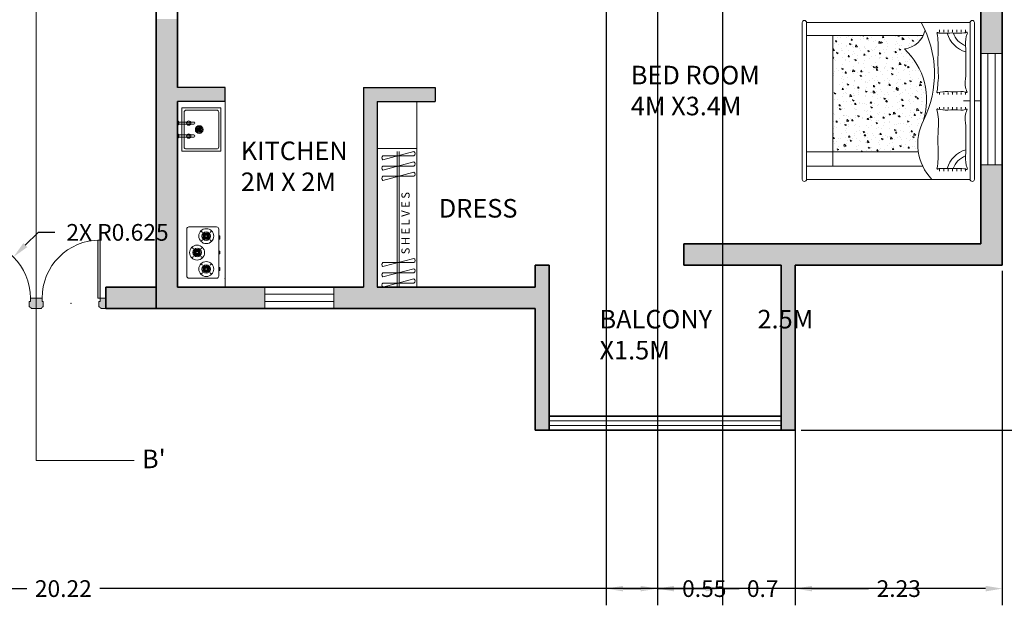
# Model space of a CAD drawing. Units: metres. Extents: x 2031 to 2061.8, y 1886.4 to 1909.8.
# Tile 7 of 10: x 2045.9 to 2056.5, y 1886.4 to 1892.7. Entities that reach past the tile are written whole.
import ezdxf

# ---------------------------------------------------------------- set-up
doc = ezdxf.new("R2010")
doc.units = ezdxf.units.M
for name, color, linetype, lineweight in [('A-ANNO-DIMS', 2, 'Continuous', 18), ('A-ANNO-SYMB', 7, 'Continuous', 18), ('A-AREA-IDEN', 7, 'Continuous', 18), ('A-EQPM', 8, 'Continuous', 18), ('A-FLOR-CASE', 8, 'Continuous', 18), ('A-FLOR-FIXT', 8, 'Continuous', 18), ('A-WALL-PATT', 252, 'Continuous', 13), ('doors & windows', 30, 'Continuous', 18), ('furniture', 24, 'Continuous', 13), ('grills', 5, 'Continuous', 13), ('inner walls', 4, 'Continuous', 25), ('windows', 30, 'Continuous', 18)]:
    doc.layers.add(name, color=color, linetype=linetype, lineweight=lineweight)
doc.layers.add('outer walls', color=1, linetype='Continuous', lineweight=35, plot=False)
doc.styles.get("Standard").update_dxf_attribs({"font": 'arial.ttf'})
doc.dimstyles.get("Standard").update_dxf_attribs({"dimtxt": 0.18, "dimasz": 0.18, "dimexe": 0.18, "dimexo": 0.0625, "dimgap": 0.09, "dimtad": 0, "dimtih": 1, "dimtoh": 1, "dimdec": 4, "dimzin": 0, "dimdsep": 46, "dimtxsty": 'Standard', "dimcen": 0.09, "dimadec": 0, "dimazin": 0, "dimtfac": 1, "dimtdec": 4, "dimtofl": 0, "dimtmove": 0, "dimatfit": 3, "dimfxl": 1, "dimtolj": 1, "dimtzin": 0, "dimarcsym": 0})

# ---------------------------------------------------------------- blocks, each defined once
blk = doc.blocks.new('sink')
for p, q in [((0, 0), (-22.00000000000001, 0)), ((0, 0), (0, 0)), ((-20.00000000000023, -2.999999999999995), (-2.000000000000178, -3)), ((-19.99999999999959, -22.99999999999988), (-20.00000000000023, -2.999999999999995)), ((-18.00000000000017, -3.999999999999996), (-4.000000000000113, -3.999999999999999)), ((-2.000000000000178, -3), (-1.999999999999543, -22.99999999999988)), ((-18.99999999999966, -20.99999999999994), (-19.00000000000017, -4.999999999999996)), ((-3.000000000000114, -5), (-2.999999999999607, -20.99999999999988)), ((-2.4e-15, -8.999999999999813), (-2.9e-15, -10.99999999999981)), ((-0.5000000000000026, -9.499999999999813), (-7.500000000000004, -9.499999999999812)), ((-0.5000000000000028, -10.49999999999981), (-7.500000000000004, -10.49999999999981)), ((-0.5000000000000026, -9.499999999999813), (-0.5000000000000028, -10.49999999999981)), ((-0.500000000000004, -15.49999999999981), (-7.500000000000005, -15.49999999999981)), ((-0.5000000000000044, -16.49999999999981), (-7.500000000000005, -16.49999999999981)), ((-0.500000000000004, -15.49999999999981), (-0.5000000000000044, -16.49999999999981)), ((-3.9e-15, -14.99999999999981), (-4.4e-15, -16.99999999999981)), ((-17.99999999999966, -21.99999999999988), (-3.999999999999607, -21.99999999999989)), ((-19.99999999999959, -22.99999999999988), (-1.999999999999543, -22.99999999999988))]:
    blk.add_line(p, q)
for centre, radius in [((-5.180961460384426, -9.999999999999812), 1), ((-10.00000000000014, -12.99999999999968), 1.794435724606955), ((-10.00000000000014, -12.99999999999968), 1.294435724606955), ((-10.66093109696162, -12.61841125325318), 0.25), ((-10.66093109696162, -13.38158874674618), 0.25), ((-10.00000000000014, -12.23682250650668), 0.25), ((-10.00000000000014, -12.99999999999968), 0.25), ((-10.00000000000014, -13.76317749349269), 0.25), ((-9.33906890303867, -12.61841125325318), 0.25), ((-9.33906890303867, -13.38158874674618), 0.25), ((-5.180961460384426, -9.999999999999812), 0.5), ((-5.180961460384427, -15.99999999999981), 1), ((-5.180961460384427, -15.99999999999981), 0.5)]:
    blk.add_circle(centre, radius)
for centre, radius, start, end in [((-18.00000000000017, -4.999999999999996), 1, 89.99999999999999, 180), ((-4.000000000000115, -5), 1, 0, 89.99999999999999), ((0.010449978117122, -9.510449978116938), 0.5105569333604445, 91.17280055555744, 178.8271994444424), ((-7.500000000000004, -9.999999999999812), 0.5, 89.99999999999999, 270), ((0.0104499781171218, -10.48955002188269), 0.5105569333604445, 181.1728005555574, 268.8271994444423), ((-7.500000000000005, -15.99999999999981), 0.5, 89.99999999999999, 270), ((0.0104499781171206, -15.51044997811693), 0.5105569333604445, 91.17280055555744, 178.8271994444424), ((0.0104499781171203, -16.48955002188269), 0.5105569333604445, 181.1728005555573, 268.8271994444423), ((-17.99999999999966, -20.99999999999988), 1, 180, 270), ((-3.999999999999607, -20.99999999999988), 1, 270, 0)]:
    blk.add_arc(centre, radius, start, end)
blk = doc.blocks.new('stove')
at = {"layer": 'furniture'}
h = blk.add_hatch(dxfattribs=at)
h.set_pattern_fill('HEX', color=256, angle=180, style=0)
h.set_pattern_definition([(360, (23.99999999999982, 24.99999999999816), (1e-16, 0.216506351), [0.125, -0.25]), (119.9999999999999, (23.99999999999982, 24.99999999999816), (-0.1875000000466704, -0.1082531754999999), [0.1249999999999998, -0.2499999999999996]), (59.99999999999994, (24.12499999999982, 24.99999999999816), (-0.1875000000466704, 0.1082531755000001), [0.125, -0.25])])
h.paths.add_polyline_path([(10.36428182591571, 19.71316705046143, 1), (7.364281825915714, 19.71316705046143, 1)])
h.paths.add_polyline_path([(9.364281825915715, 19.71316705046143, -1), (8.364281825915715, 19.71316705046143, -1)], flags=16)
h = blk.add_hatch(dxfattribs=at)
h.set_pattern_fill('HEX', color=256, angle=180, style=0)
h.set_pattern_definition([(180, (-2.000000000000001, 6.713167050462818), (-1e-16, -0.216506351), [0.125, -0.25]), (300, (-2.000000000000001, 6.713167050462818), (0.1875000000466704, 0.1082531754999999), [0.1249999999999999, -0.2499999999999998]), (239.9999999999999, (-2.125000000000001, 6.713167050462818), (0.1875000000466704, -0.1082531755000001), [0.125, -0.25])])
h.paths.add_polyline_path([(14.6357181740841, 11.99999999999954, 1), (11.6357181740841, 11.99999999999954, 1)])
h.paths.add_polyline_path([(12.6357181740841, 11.99999999999954, -1), (13.6357181740841, 11.99999999999954, -1)], flags=16)
h = blk.add_hatch(dxfattribs=at)
h.set_pattern_fill('HEX', color=256, angle=180, style=0)
h.set_pattern_definition([(360, (23.99999999999982, -0.9999999999999342), (-1e-16, -0.216506351), [0.125, -0.25]), (239.9999999999999, (23.99999999999982, -0.9999999999999342), (-0.1875000000466704, 0.1082531755), [0.1249999999999999, -0.2499999999999998]), (300, (24.12499999999982, -0.9999999999999342), (-0.1875000000466704, -0.1082531755), [0.125, -0.2499999999999999])])
h.paths.add_polyline_path([(10.36428182591571, 4.2868329495368, 1), (7.364281825915714, 4.2868329495368, 1)])
h.paths.add_polyline_path([(9.364281825915715, 4.2868329495368, -1), (8.364281825915715, 4.2868329495368, -1)], flags=16)
for p, q in [((4.000000000000007, 23.99999999999909), (17, 23.99999999999908)), ((3.000000000000007, 19.86017834974973), (2.500000000000003, 19.86017834974973)), ((2.500000000000003, 19.86017834974973), (2.500000000000003, 18.36017834974973)), ((3, 1.000000000000003), (3.000000000000007, 22.99999999999909)), ((6.389408091762671, 22.18804078461422), (7.09651487294905, 21.48093400342751)), ((10.6320487788818, 21.48093400342809), (11.33915556006851, 22.18804078461447)), ((18, 22.99999999999908), (18, 0.9999999999991327)), ((2.500000000000003, 18.36017834974973), (3.000000000000003, 18.36017834974973)), ((6.389408091762675, 17.23829331630864), (7.096514872949061, 17.94540009749535)), ((10.63204877888179, 17.94540009749477), (11.3391555600685, 17.23829331630838)), ((11.36795122111803, 13.7677669529662), (10.66084443993131, 14.47487373415259)), ((15.61059190823715, 14.47487373415233), (14.90348512705075, 13.76776695296562)), ((2.500000000000003, 12.64999999999954), (2.500000000000003, 11.34999999999955)), ((3.000000000000003, 12.64999999999954), (2.500000000000003, 12.64999999999954)), ((2.500000000000003, 11.34999999999955), (3.000000000000003, 11.34999999999955)), ((11.36795122111803, 10.23223304703288), (10.66084443993131, 9.525126265846504)), ((15.61059190823714, 9.525126265846753), (14.90348512705077, 10.23223304703346)), ((2.500000000000003, 4.936832949536799), (2.500000000000003, 3.636832949536802)), ((3.000000000000003, 4.936832949536799), (2.500000000000003, 4.936832949536799)), ((6.389408091762671, 6.761706683689592), (7.096514872949061, 6.054599902502877)), ((10.63204877888178, 6.05459990250346), (11.3391555600685, 6.761706683689842)), ((2.500000000000003, 3.636832949536802), (3.000000000000003, 3.636832949536802)), ((16.99999999999994, -8.669e-13), (3.999999999999946, 3.6e-15)), ((6.389408091762668, 1.811959215384014), (7.096514872949043, 2.519065996570723)), ((10.63204877888179, 2.519065996570138), (11.3391555600685, 1.81195921538376))]:
    blk.add_line(p, q, dxfattribs=at)
for centre, radius in [((8.864281825915715, 19.71316705046143), 3.499999999999999), ((8.864281825915715, 19.71316705046143), 1.999999999999999), ((8.864281825915715, 19.71316705046143), 1.5), ((8.864281825915715, 19.71316705046143), 0.5000000000000004), ((13.1357181740841, 11.99999999999954), 3.499999999999999), ((13.1357181740841, 11.99999999999954), 1.999999999999999), ((13.1357181740841, 11.99999999999954), 1.5), ((13.1357181740841, 11.99999999999954), 0.5000000000000004), ((8.864281825915715, 4.286832949536801), 3.499999999999999), ((8.864281825915715, 4.2868329495368), 1.999999999999999), ((8.864281825915715, 4.2868329495368), 1.5), ((8.864281825915715, 4.2868329495368), 0.5000000000000004)]:
    blk.add_circle(centre, radius, dxfattribs=at)
for centre, start, end in [((4.000000000000007, 22.99999999999909), 90, 180), ((17, 22.99999999999908), 0, 90), ((4, 1.000000000000003), 180, 269.9999999999968), ((17, 0.9999999999991331), 269.9999999999968, 0)]:
    blk.add_arc(centre, 1, start, end, dxfattribs=at)
at = {"layer": 'furniture', "ltscale": 9}
blk.add_point((0, 0), dxfattribs=at)
blk = doc.blocks.new('hangers')
at = {"layer": 'furniture'}
for p, q in [((1.8e-15, 16.5), (4.000000000000001, 1.5)), ((2.000000000000001, 16.5), (2.000000000000001, 1.5)), ((5.000000000000001, 16.5), (9.000000000000002, 1.5)), ((7.000000000000001, 16.5), (7.000000000000001, 1.5)), ((10, 16.5), (14, 1.5)), ((12, 16.5), (12, 1.5)), ((52, 16.5), (56, 1.5)), ((54, 16.5), (54, 1.5)), ((57, 16.5), (61, 1.5)), ((59, 16.5), (59, 1.5)), ((62, 16.5), (66, 1.5)), ((64, 16.5), (64, 1.5)), ((66, 9.5), (1.8e-15, 9.5)), ((1.8e-15, 8.5), (66, 8.5))]:
    blk.add_line(p, q, dxfattribs=at)
for centre, radius, start, end in [((1.000000000000001, 15.6218374153911), 1.33085293139661, 41.28839256573093, 138.711607434269), ((6.000000000000001, 15.6218374153911), 1.33085293139661, 41.28839256573093, 138.711607434269), ((11, 15.6218374153911), 1.33085293139661, 41.28839256573093, 138.711607434269), ((53, 15.6218374153911), 1.33085293139661, 41.28839256573107, 138.7116074342689), ((58, 15.6218374153911), 1.33085293139661, 41.28839256573107, 138.7116074342689), ((63, 15.6218374153911), 1.33085293139661, 41.28839256573107, 138.7116074342689), ((3.000000000000001, 1.915335972440686), 1.082822224561017, 202.5548696812492, 337.4451303187508), ((8.000000000000002, 1.915335972440686), 1.082822224561017, 202.5548696812492, 337.4451303187508), ((13, 1.915335972440686), 1.082822224561017, 202.5548696812492, 337.4451303187508), ((55, 1.915335972440686), 1.082822224561017, 202.5548696812491, 337.4451303187509), ((60, 1.915335972440686), 1.082822224561017, 202.5548696812491, 337.4451303187509), ((65, 1.915335972440686), 1.082822224561017, 202.5548696812491, 337.4451303187509)]:
    blk.add_arc(centre, radius, start, end, dxfattribs=at)
blk.add_point((0, 0), dxfattribs=at)
blk.add_text('S H E L V E S', height=4, dxfattribs=at).set_placement((15.9969173169515, 3.475366291579639))
blk = doc.blocks.new('bed')
at = {"layer": 'furniture'}
h = blk.add_hatch(dxfattribs=at)
h.set_pattern_fill('AR-CONC', color=256, angle=-90.00000000000003, style=0)
h.set_pattern_definition([(320, (0, 2.380000000001032), (-0.6275213498259539, -7.172601826007534), [0.75, -8.25]), (265, (0, 2.380000000001032), (7.521921337000119, 1.387513336129997), [0.6, -6.599999999999999]), (10.45139999999999, (-0.0522933999999964, 1.782283200001032), (6.894395420609534, -5.785093817140218), [0.6374019000000001, -7.011421119999999]), (316.1842, (2, 2.380000000001032), (-1.655190143290184, -10.67241048625644), [1.125, -12.375]), (6.635599999999979, (1.862066929999997, 1.490632550001038), (9.741178709004412, -9.346627055487035), [0.956102879999999, -10.51712999999998]), (261.1842, (2, 2.380000000001032), (9.741186009253243, -9.346619451336275), [0.8999999999999989, -9.899999999999984]), (291, (1.5, 1.380000000001032), (-4.02618890665339, -5.969070521184614), [0.75, -8.25]), (236, (1.5, 1.380000000001032), (7.251500450468529, -2.433153319215819), [0.6, -6.599999999999999]), (341.4514, (1.164483939999996, 0.8825776700010266), (3.22530496709952, -8.402226285814901), [0.6374019000000001, -7.011421119999999]), (307.4999999999999, (0, 2.380000000001032), (3.328938538313114, -0.121598553172908), [0, -6.519999999999999, 0, -6.7, 0, -6.625]), (277.5, (0, 2.380000000001032), (3.944117118823601, -2.630695374421487), [0, -3.819999999999999, 0, -6.37, 0, -2.524999999999999]), (237.5, (0, 4.610000000001036), (-0.2255487173438, -5.33822436172409), [0, -2.5, 0, -7.799999999999999, 0, -10.35]), (227.5, (0, 5.610000000001036), (1.001049823323174, -5.831861693423862), [0, -3.25, 0, -5.179999999999999, 0, -7.349999999999999])])
h.paths.add_polyline_path([(30.01221964123038, -67.99999999999999), (30.01221964123036, -26.4972098666525, 0.2630430180581192), (23.90476957024844, -35.1500155485824, 0.2934236934375176), (-9.177957282599145, -26.46678060096597, -0.1566832162072435), (-23.39221964123496, -28.71851562074189), (-23.39221964123494, -67.99999999999999)])
for p, q in [((0, -3), (0, 0)), ((36.01221964123033, -3), (-36.01221964123033, -3)), ((-36.01221964123033, -5.000000000000028), (-36.01221964123027, -80)), ((36.01221964123033, -5.000000000000042), (-36.01221964123033, -5.000000000000028)), ((-31.23716250644156, -7.067621994530554), (-32.23716250644157, -7.067621994530554)), ((-3.810600647213163, -7.067621994530554), (-2.810600647213163, -7.067621994530554)), ((0, -8.000000000000043), (0, -5.000000000000042)), ((3.894900133777696, -7.067621994530526), (2.894900133777696, -7.067621994530526)), ((31.62837541028949, -7.067621994530526), (32.62837541028949, -7.067621994530526)), ((36.01221964123039, -79.99999999999999), (36.01221964123033, -5.000000000000042)), ((-31.23716250644156, -9.067621994530555), (-32.23716250644157, -9.067621994530555)), ((-31.23716250644156, -11.06762199453055), (-32.23716250644157, -11.06762199453055)), ((-31.23716250644156, -13.06762199453055), (-32.23716250644157, -13.06762199453055)), ((-3.810600647213163, -9.067621994530555), (-2.810600647213163, -9.067621994530555)), ((-3.810600647213163, -11.06762199453055), (-2.810600647213163, -11.06762199453055)), ((-3.810600647213163, -13.06762199453055), (-2.810600647213163, -13.06762199453055)), ((3.894900133777696, -9.067621994530526), (2.894900133777696, -9.067621994530526)), ((3.894900133777696, -11.06762199453052), (2.894900133777696, -11.06762199453052)), ((3.894900133777696, -13.06762199453052), (2.894900133777696, -13.06762199453052)), ((31.62837541028949, -9.067621994530526), (32.62837541028949, -9.067621994530526)), ((31.62837541028949, -11.06762199453052), (32.62837541028949, -11.06762199453052)), ((31.62837541028949, -13.06762199453052), (32.62837541028949, -13.06762199453052)), ((-31.23716250644156, -15.06762199453055), (-32.23716250644157, -15.06762199453055)), ((-31.23716250644156, -17.06762199453055), (-32.23716250644157, -17.06762199453055)), ((-3.810600647213163, -15.06762199453055), (-2.810600647213163, -15.06762199453055)), ((-3.810600647213163, -17.06762199453055), (-2.810600647213163, -17.06762199453055)), ((3.894900133777696, -15.06762199453052), (2.894900133777696, -15.06762199453052)), ((3.894900133777696, -17.06762199453052), (2.894900133777696, -17.06762199453052)), ((31.62837541028949, -15.06762199453052), (32.62837541028949, -15.06762199453052)), ((31.62837541028949, -17.06762199453052), (32.62837541028949, -17.06762199453052)), ((-31.23716250644156, -19.06762199453055), (-32.23716250644157, -19.06762199453055)), ((-3.810600647213163, -19.06762199453055), (-2.810600647213163, -19.06762199453055)), ((3.894900133777696, -19.06762199453052), (2.894900133777696, -19.06762199453052)), ((31.62837541028949, -19.06762199453052), (32.62837541028949, -19.06762199453052)), ((-36.01221964123027, -80), (36.01221964123039, -79.99999999999997)), ((-36.01221964123027, -82), (36.01221964123039, -82))]:
    blk.add_line(p, q, dxfattribs=at)
at = {"layer": 'furniture', "ltscale": 5}
blk.add_line((-30.0122196412303, -26.65900214866815), (-30.01221964123028, -80), dxfattribs=at)
at = {"layer": 'furniture', "ltscale": 7}
blk.add_line((30.01221964123039, -79.99999999999999), (30.01221964123036, -26.4972098666525), dxfattribs=at)
at = {"layer": 'furniture', "ltscale": 0.3}
for p, q in [((-23.39221964123493, -80.00000000000003), (-23.39221964123496, -28.71851562074188)), ((-30.01221964123028, -67.99999999999999), (30.01221964123039, -67.99999999999999))]:
    blk.add_line(p, q, dxfattribs=at)
at = {"layer": 'furniture'}
for centre, radius, start, end in [((-35.95310404783035, -4.000000000000014), 1.001745802777857, 93.38313670775338, 266.6168632922466), ((35.95310404783047, -4.000000000000014), 1.001745802777857, 273.3831367077534, 86.61686329224663), ((-31.09685452420217, -6.56812628935117), 0.3815901177143176, 35.89755946985184, 208.6271807330242), ((-44.4434251214767, -13.85312857714783), 14.82374463825802, 27.16285943351717, 28.62718073212637), ((-46.75951437957865, -9.65138206848897), 15.71579241958107, 357.4803608088326, 9.395608387614068), ((-34.45294545533051, -3.506108501804959), 9.853247350176973, 289.8695209624031, 338.9842964810487), ((-34.45294545533051, -3.506108501804959), 12.47479548168961, 286.0319050224358, 344.1205283884622), ((-26.34909713879518, 6.677823774407073), 13.75788850886336, 251.1782289026713, 273.3982224065857), ((-18.01528168092849, -163.5963416214672), 156.7209082093599, 87.00321809951629, 92.74968346925495), ((-8.031939823939297, 2.030581047412752), 9.294330538692307, 258.8960367609226, 294.7184225587751), ((0.254091396095987, -8.800915214962217), 4.494229367051207, 159.014640107615, 186.2730421081171), ((-4.029449448298862, -6.668977911985379), 0.2818061021667602, 335.7259061638442, 114.3030308467571), ((3.223958981487498, -9.94006998173215), 7.675076275868892, 155.7259061638442, 159.0146401085631), ((4.113748934860268, -6.668977911985379), 0.2818061021635516, 65.69696915417202, 204.2740938370052), ((-3.139659494904833, -9.940069981732137), 7.675076275868892, 20.98535989143595, 24.27409383615427), ((-0.1697919095242355, -8.800915214962217), 4.494229367051207, 353.7269578918828, 20.98535989238499), ((8.116239310533615, 2.030581047735168), 9.294330539002221, 245.2815774418415, 281.1039632384965), ((18.09958116748922, -163.5963416214399), 156.7209082093326, 87.2503165307418, 92.99678190048373), ((34.53724494190226, -3.506108501789682), 12.47479548168961, 195.8794716115377, 253.9680949775642), ((34.53724494190226, -3.506108501789682), 9.853247350176973, 201.0157035189505, 250.1304790375968), ((26.43339662535652, 6.677823774423444), 13.75788850886336, 266.6017775934111, 288.8217710973251), ((31.18115401076358, -6.568126289351184), 0.3815901177179044, 331.3728192669758, 144.1024405301472), ((46.84381386614001, -9.651382068520647), 15.71579241958353, 170.6043916115409, 182.5196391911672), ((44.52772460803806, -13.85312857714784), 14.82374463825802, 151.3728192678729, 152.8371405664821), ((-28.61556435462791, 31.03444768063454), 42.31456350822244, 266.4835611990511, 266.6487421238194), ((54.88285648445511, -13.16191061182081), 85.98801403775587, 178.1208768196816, 183.3613129440673), ((-32.81622258778788, -12.43616332427339), 28.77528664700029, 354.3784002715227, 6.27304210895588), ((32.90052207435963, -12.43616332427341), 28.77528664700055, 173.7269578910441, 185.6215997284773), ((-54.79855699787332, -13.1619106118885), 85.98801403775471, 356.6386870559327, 1.87912318031836), ((28.69986384117891, 31.03444768073385), 42.31456350831875, 273.3512578762066, 273.5164388009489), ((12.27920019974715, -16.10835590841725), 16.48064095036883, 177.0317121189266, 192.8677860199701), ((-12.19490071317551, -16.10835590841725), 16.48064095036894, 347.1322139800299, 2.968287881073314), ((-19.78970084288576, -5.469494448941333), 23.52647715105876, 226.4060518471351, 297.4441169484015), ((-31.05019458355673, -19.91479358257859), 0.2912925215689113, 147.6219291273817, 311.93432899363), ((-33.19532486499685, -18.55460390606353), 2.248727139855352, 327.6219291288709, 339.224552802207), ((-34.12771521855714, -18.41167218428833), 3.177308659740759, 342.7808628527732, 3.755021134780372), ((-24.39731400277299, -58.0065508966982), 38.42172354635978, 93.51643880178425, 99.67664784205135), ((-24.51665474671893, -56.06449133928439), 36.47600066328987, 86.48356119821578, 93.51643880178425), ((-18.48842024981553, 70.49496359167773), 90.23180174042126, 267.5920770069633, 273.6328801943956), ((-10.30534078399284, -44.95285539311296), 25.51674577343078, 75.95197577712642, 95.54518109318596), ((12.50744191168894, -69.71437404891591), 48.3828132966499, 60.93454900685955, 116.3226601669859), ((-3.947726608991956, -19.99033763805275), 0.2654728058058112, 231.9004795059564, 52.89022406852256), ((4.032026095563765, -19.99033763805275), 0.2654728058058112, 127.1097759314774, 308.0995204940429), ((7.570216687580227, -34.67789736270967), 14.86666553287629, 87.39755039330738, 103.1191401867811), ((11.43897390287765, -34.80624327566366), 15.31635237680183, 84.69404282866213, 102.035481886755), ((18.57271973638731, 70.4949635916777), 90.23180174042125, 266.3671198056044, 272.4079229930367), ((24.6009542333012, -56.0644913392844), 36.47600066328987, 86.48356119821578, 93.51643880178425), ((24.48161348934542, -58.00655089669821), 38.42172354635978, 80.32335215794863, 86.48356119821578), ((31.13449407013883, -19.91479358255678), 0.2912925215689113, 228.06567100637, 32.37807087261824), ((34.21201470513921, -18.41167218428845), 3.177308659740705, 176.2449788652196, 197.2191371472267), ((33.27962435157895, -18.55460390604825), 2.248727139855352, 200.775447197793, 212.378070871129), ((0.602167516954296, -56.56840710701565), 31.65057281321388, 42.58740832788977, 108.5033645785765), ((34.6132349005153, -36.22659364526982), 10.76244628919441, 101.1719081394, 174.2590453022261), ((-35.95310404783035, -81), 1.001745802777857, 93.38313670775338, 266.6168632922466), ((35.95310404783044, -81), 1.001745802777857, 273.3831367077534, 86.61686329224663)]:
    blk.add_arc(centre, radius, start, end, dxfattribs=at)
blk = doc.blocks.new('D2')
at = {"layer": 'doors & windows'}
h = blk.add_hatch(dxfattribs=at)
h.set_pattern_fill('DOTS', color=256, scale=2, angle=180, style=0)
h.set_pattern_definition([(180, (0, -3.999999999998181), (-0.0625, -0.125), [0, -0.125])])
h.paths.add_polyline_path([(2.5, 1.819e-12), (3.5, 1.819e-12), (3.500000000001818, 24.97999199359535, 0.0100030022021123), (2.500000000001818, 25.00000000000182)])
h = blk.add_hatch(dxfattribs=at)
h.set_pattern_fill('DOTS', color=256, scale=2, angle=180, style=0)
h.set_pattern_definition([(180, (0, 0), (-0.0625, -0.125), [0, -0.125])])
edge = h.paths.add_edge_path()
edge.add_line((27.50000000000182, 1.819e-12), (27.50000000000182, -1.499999999998181))
edge.add_line((27.50000000000182, -1.499999999998181), (27.00000000000157, -1.499999999998181))
edge.add_line((27.00000000000157, -1.499999999998181), (27.00000000000039, -3.749999999998181))
edge.add_line((27.00000000000039, -3.749999999998181), (27.25, -3.749999999998181))
edge.add_arc((27.75893604593965, -3.741063954058532), 0.5090144907305875, 181.0059124648427, 268.9940875351573)
edge.add_line((27.75, -4.249999999998181), (27.75, -4.499999999998181))
edge.add_line((27.75, -4.499999999998181), (30.00000000000182, -4.499999999998181))
edge.add_line((30.00000000000182, -4.499999999998181), (30.00000000000182, 0))
edge.add_line((30.00000000000182, 0), (27.50000000000182, 1.819e-12))
edge = h.paths.add_edge_path()
edge.add_line((2.5, -1.499999999998181), (2.5, 1.819e-12))
edge.add_line((2.5, 1.819e-12), (1.819e-12, 0))
edge.add_line((1.819e-12, 0), (0, -4.499999999998181))
edge.add_line((0, -4.499999999998181), (2.250000000001548, -4.499999999998181))
edge.add_line((2.250000000001548, -4.499999999998181), (2.250000000001548, -4.249999999998181))
edge.add_arc((2.2410639540619, -3.741063954058532), 0.5090144907305875, 271.0059124648427, 358.9940875351573)
edge.add_line((2.750000000001548, -3.749999999998181), (3, -3.749999999998181))
edge.add_line((3, -3.749999999998181), (3, -1.499999999998181))
edge.add_line((3, -1.499999999998181), (2.5, -1.499999999998181))
for p, q in [((1.819e-12, 0), (0, -4.499999999998181)), ((30.00000000000182, 0), (30.00000000000182, -4.499999999998181))]:
    blk.add_line(p, q)
blk.add_lwpolyline([(3.5, 1.819e-12), (3.500000000001818, 25.00000000000182), (2.500000000001818, 25.00000000000182), (2.5, 1.819e-12)], close=True, dxfattribs=at)
for points in [[(3, -3.749999999998181), (3, -1.499999999998181), (2.5, -1.499999999998181), (2.5, 1.819e-12), (1.819e-12, 0)], [(27.00000000000039, -3.749999999998181), (27.00000000000182, -1.499999999998181), (27.50000000000182, -1.499999999998181), (27.50000000000182, 1.819e-12), (30, 0)], [(0, -4.499999999998181), (2.250000000001548, -4.499999999998181)], [(30, -4.499999999998181), (27.75, -4.499999999998181)]]:
    blk.add_lwpolyline(points, dxfattribs=at)
for points in [[(2.250000000001548, -4.499999999998181), (2.250000000001548, -4.249999999998181, 0.4039662087126686), (2.750000000001548, -3.749999999998181), (3.000000000001548, -3.749999999998181)], [(27.75, -4.499999999998181), (27.75, -4.249999999998181, -0.4039662087126686), (27.25, -3.749999999998181), (27, -3.749999999998181)]]:
    blk.add_lwpolyline(points, format="xyb", dxfattribs=at)
at = {"layer": 'doors & windows', "ltscale": 6}
blk.add_arc((2.5, 1.819e-12), 25, 0, 90, dxfattribs=at)
at = {"layer": 'doors & windows'}
blk.add_point((15, -2.24999999999909), dxfattribs=at)
blk = doc.blocks.new('WIN-1200')
for p, q in [((0.2299999999995634, 1.200000000000045), (-4.547e-13, 1.199999999999818)), ((0.0750000000007276, -2.274e-13), (0.0749999999995907, 1.200000000000045)), ((0.1550000000006548, -2.274e-13), (0.154999999999518, 1.200000000000045)), ((0.2300000000007003, 0), (6.821e-13, -2.274e-13))]:
    blk.add_line(p, q)
blk = doc.blocks.new('BALCONY-GUARD-2500')
for p, q in [((4.547e-13, 0.0500000000010914), (2.5, 0.0500000000006367)), ((4.547e-13, 6.821e-13), (2.5, 4.547e-13))]:
    blk.add_line(p, q)
blk = doc.blocks.new('*D44')
at = {"layer": 'A-ANNO-DIMS', "color": 0, "lineweight": -2, "transparency": 16777216}
for p, q in [((2036.232783, 1900.719895), (2036.232783, 1886.390195)), ((2056.453886, 1889.9931), (2056.453886, 1886.390195)), ((2036.412783, 1886.570195), (2045.94901662824, 1886.570195)), ((2056.273886, 1886.570195), (2046.73765237176, 1886.570195))]:
    blk.add_line(p, q, dxfattribs=at)
at = {"layer": 'A-ANNO-DIMS', "color": 0, "transparency": 16777216}
for points in [[(2036.412783, 1886.600195), (2036.412783, 1886.540195), (2036.232783, 1886.570195)], [(2056.273886, 1886.600195), (2056.273886, 1886.540195), (2056.453886, 1886.570195)]]:
    blk.add_solid(points, dxfattribs=at)
at = {"layer": 'Defpoints', "color": 0, "transparency": 16777216}
for p in [(2036.232783, 1900.782395), (2056.453886, 1890.0556), (2056.453886, 1886.570195)]:
    blk.add_point(p, dxfattribs=at)
at = {"layer": 'A-ANNO-DIMS', "color": 0, "transparency": 16777216, "insert": (2046.3433345, 1886.570195), "char_height": 0.18, "attachment_point": 5}
blk.add_mtext('\\A1;20.22', dxfattribs=at)
blk = doc.blocks.new('*D45')
at = {"layer": 'A-ANNO-DIMS', "color": 0, "lineweight": -2, "transparency": 16777216}
for p, q in [((2047.556386000001, 1907.081203000001), (2061.614374000002, 1907.081203000001)), ((2061.434374000002, 1906.901203000001), (2061.434374000002, 1897.862029637791)), ((2061.434374000002, 1888.459050000001), (2061.434374000002, 1897.498223362211)), ((2054.286386000001, 1888.279050000001), (2061.614374000002, 1888.279050000001))]:
    blk.add_line(p, q, dxfattribs=at)
at = {"layer": 'A-ANNO-DIMS', "color": 0, "transparency": 16777216}
for points in [[(2061.404374000002, 1906.901203000001), (2061.464374000002, 1906.901203000001), (2061.434374000002, 1907.081203000001)], [(2061.404374000002, 1888.459050000001), (2061.464374000002, 1888.459050000001), (2061.434374000002, 1888.279050000001)]]:
    blk.add_solid(points, dxfattribs=at)
at = {"layer": 'Defpoints', "color": 0, "transparency": 16777216}
for p in [(2047.493886000001, 1907.081203000001), (2061.434374000002, 1907.081203000001), (2054.223886000001, 1888.279050000001)]:
    blk.add_point(p, dxfattribs=at)
at = {"layer": 'A-ANNO-DIMS', "color": 0, "transparency": 16777216, "insert": (2061.434374000002, 1897.6801265), "char_height": 0.18, "attachment_point": 5}
blk.add_mtext('\\A1;18.802', dxfattribs=at)
blk = doc.blocks.new('*D56')
at = {"layer": 'A-ANNO-DIMS', "color": 0, "lineweight": -2, "transparency": 16777216}
for p, q in [((2054.223886, 1889.9931), (2054.223886, 1886.390195)), ((2056.453886, 1889.9931), (2056.453886, 1886.390195)), ((2054.403886, 1886.570195), (2055.013572221009, 1886.570195)), ((2056.273886, 1886.570195), (2055.664199778991, 1886.570195))]:
    blk.add_line(p, q, dxfattribs=at)
at = {"layer": 'A-ANNO-DIMS', "color": 0, "transparency": 16777216}
for points in [[(2054.403886, 1886.600195), (2054.403886, 1886.540195), (2054.223886, 1886.570195)], [(2056.273886, 1886.600195), (2056.273886, 1886.540195), (2056.453886, 1886.570195)]]:
    blk.add_solid(points, dxfattribs=at)
at = {"layer": 'Defpoints', "color": 0, "transparency": 16777216}
for p in [(2054.223886, 1890.0556), (2056.453886, 1890.0556), (2056.453886, 1886.570195)]:
    blk.add_point(p, dxfattribs=at)
at = {"layer": 'A-ANNO-DIMS', "color": 0, "transparency": 16777216, "insert": (2055.338886, 1886.570195), "char_height": 0.18, "attachment_point": 5}
blk.add_mtext('\\A1;2.23', dxfattribs=at)
blk = doc.blocks.new('*D62')
at = {"layer": 'A-ANNO-DIMS', "color": 0, "lineweight": -2, "transparency": 16777216}
for p, q in [((2052.190038, 1893.772326), (2052.190038, 1886.390195)), ((2052.740231, 1893.6231), (2052.740231, 1886.390195)), ((2052.370038, 1886.570195), (2052.560231000001, 1886.570195)), ((2052.740231, 1886.570195), (2052.920231, 1886.570195))]:
    blk.add_line(p, q, dxfattribs=at)
at = {"layer": 'A-ANNO-DIMS', "color": 0, "transparency": 16777216}
for points in [[(2052.370038, 1886.600195), (2052.370038, 1886.540195), (2052.190038, 1886.570195)], [(2052.560231000001, 1886.600195), (2052.560231000001, 1886.540195), (2052.740231, 1886.570195)]]:
    blk.add_solid(points, dxfattribs=at)
at = {"layer": 'Defpoints', "color": 0, "transparency": 16777216}
for p in [(2052.190038, 1893.834826), (2052.740231, 1893.6856), (2052.740231, 1886.570195)]:
    blk.add_point(p, dxfattribs=at)
at = {"layer": 'A-ANNO-DIMS', "color": 0, "transparency": 16777216, "insert": (2053.244685297408, 1886.570195), "char_height": 0.18, "attachment_point": 5}
blk.add_mtext('\\A1;0.55', dxfattribs=at)
blk = doc.blocks.new('*D63')
at = {"layer": 'A-ANNO-DIMS', "color": 0, "lineweight": -2, "transparency": 16777216}
for p, q in [((2052.740231, 1893.6231), (2052.740231, 1886.390195)), ((2053.440231, 1893.623873), (2053.440231, 1886.390195)), ((2052.920231, 1886.570195), (2053.260231, 1886.570195)), ((2053.440231, 1886.570195), (2053.620231, 1886.570195))]:
    blk.add_line(p, q, dxfattribs=at)
at = {"layer": 'A-ANNO-DIMS', "color": 0, "transparency": 16777216}
for points in [[(2052.920231, 1886.600195), (2052.920231, 1886.540195), (2052.740231, 1886.570195)], [(2053.260231, 1886.600195), (2053.260231, 1886.540195), (2053.440231, 1886.570195)]]:
    blk.add_solid(points, dxfattribs=at)
at = {"layer": 'Defpoints', "color": 0, "transparency": 16777216}
for p in [(2052.740231, 1893.6856), (2053.440231, 1893.686373), (2053.440231, 1886.570195)]:
    blk.add_point(p, dxfattribs=at)
at = {"layer": 'A-ANNO-DIMS', "color": 0, "transparency": 16777216, "insert": (2053.874085024557, 1886.570195), "char_height": 0.18, "attachment_point": 5}
blk.add_mtext('\\A1;0.7', dxfattribs=at)
blk = doc.blocks.new('*D65')
at = {"layer": 'A-ANNO-DIMS', "color": 0, "lineweight": -2, "transparency": 16777216}
for p, q in [((2046.070887774461, 1890.408268174999), (2045.933100891741, 1890.270283483999)), ((2046.250887774462, 1890.408268174999), (2046.070887774461, 1890.408268174999)), ((2045.364289, 1889.610655), (2045.364289000001, 1889.790655)), ((2045.274289, 1889.700655), (2045.454289, 1889.700655))]:
    blk.add_line(p, q, dxfattribs=at)
at = {"layer": 'A-ANNO-DIMS', "color": 0, "transparency": 16777216}
blk.add_solid([(2045.911872477741, 1890.291481465956), (2045.954329305741, 1890.249085502042), (2045.805913, 1890.142913)], dxfattribs=at)
at = {"layer": 'Defpoints', "color": 0, "transparency": 16777216}
for p in [(2045.805913, 1890.142913), (2045.364289, 1889.700655)]:
    blk.add_point(p, dxfattribs=at)
at = {"layer": 'A-ANNO-DIMS', "color": 0, "transparency": 16777216, "insert": (2046.926317515253, 1890.408268174999), "char_height": 0.18, "attachment_point": 5}
blk.add_mtext('\\A1;2X R0.625', dxfattribs=at)

msp = doc.modelspace()

# ---------------------------------------------------------------- hatches: boundary and pattern name
at = {"layer": 'A-WALL-PATT'}
h = msp.add_hatch(color=256, dxfattribs=at)
h.dxf.hatch_style = 1
h.paths.add_polyline_path([(2051.57388605158, 1890.055599700484), (2051.42388605158, 1890.055599700485), (2051.42388605158, 1889.818154600064), (2049.72388605158, 1889.818154600064), (2049.72388605158, 1891.818397054436), (2050.347309493104, 1891.818397054436), (2050.347309493104, 1891.968397054436), (2049.573886051581, 1891.968397054436), (2049.573886051581, 1889.818154600064), (2049.254524170275, 1889.818154600064), (2049.254524170275, 1889.588154600064), (2051.42388605158, 1889.588154600064), (2051.42388605158, 1888.279049770338), (2051.57388605158, 1888.279049770338)])
h.paths.add_polyline_path([(2048.511176543873, 1889.818154600065), (2047.57388605158, 1889.818154600065), (2047.573886051581, 1891.818397054435), (2048.085735884881, 1891.818397054435), (2048.085735884881, 1891.968397054435), (2047.573886051581, 1891.968397054435), (2047.57388605158, 1892.707982727461), (2047.343886051579, 1892.707982727461), (2047.343886051578, 1889.588154600065), (2048.511176543873, 1889.588154600065)])
h.paths.add_polyline_path([(2047.57388605158, 1895.334826264002), (2047.57388605158, 1895.571212564149), (2047.34388605158, 1895.571212564149), (2047.343886051579, 1893.707982727461), (2047.57388605158, 1893.707982727461)])
h = msp.add_hatch(color=256, dxfattribs=at)
h.dxf.hatch_style = 1
h.paths.add_polyline_path([(2056.45388605158, 1891.13542096002), (2056.223886051581, 1891.13542096002), (2056.223886051581, 1890.285599700484), (2053.026296602634, 1890.285599700484), (2053.026296602634, 1890.055599700484), (2054.07388605158, 1890.055599700484), (2054.07388605158, 1888.279049770337), (2054.22388605158, 1888.279049770337), (2054.22388605158, 1890.055599700484), (2056.45388605158, 1890.055599700484)])
h.paths.add_polyline_path([(2056.45388605158, 1893.915599700484), (2054.920037956281, 1893.915599700483), (2054.920037956281, 1893.685599700484), (2056.223886051581, 1893.685599700484), (2056.223886051581, 1892.33542096002), (2056.45388605158, 1892.33542096002)])
h = msp.add_hatch(color=256, dxfattribs=at)
h.dxf.hatch_style = 1
h.paths.add_polyline_path([(2047.343886051578, 1889.818154600065), (2046.801788731911, 1889.818154600065), (2046.801788731911, 1889.588154600065), (2047.343886051578, 1889.588154600065)])

# ---------------------------------------------------------------- linework, layer by layer
at = {"layer": 'A-ANNO-SYMB'}
for q in [(2046.051788731911, 1908.279650182242), (2046.051788731911, 1887.95119549084), (2047.107009925013, 1887.95119549084)]:
    msp.add_line((2046.051788731911, 1887.95119549084), q, dxfattribs=at)
at = {"layer": 'A-FLOR-CASE', "ltscale": 0.3}
for p, q in [((2048.085735884882, 1889.818154600065), (2048.085735884881, 1891.818397054435)), ((2050.149066122807, 1889.818154600066), (2050.149066122807, 1891.818397054436))]:
    msp.add_line(p, q, dxfattribs=at)
at = {"layer": 'A-FLOR-CASE'}
msp.add_line((2050.149066122807, 1891.311337225385), (2049.72388605158, 1891.311337225385), dxfattribs=at)
at = {"layer": 'inner walls'}
for p, q in [((2048.085735884881, 1891.968397054435), (2047.57388605158, 1891.968397054435)), ((2048.085735884881, 1891.818397054435), (2048.085735884881, 1891.968397054435)), ((2049.573886051581, 1891.968397054436), (2049.573886051581, 1889.818154600065)), ((2049.573886051581, 1891.968397054436), (2050.347309493104, 1891.968397054436)), ((2050.347309493104, 1891.968397054436), (2050.347309493104, 1891.818397054436)), ((2048.085735884881, 1891.818397054435), (2047.57388605158, 1891.818397054435)), ((2049.72388605158, 1891.818397054436), (2050.347309493104, 1891.818397054436)), ((2049.72388605158, 1891.818397054436), (2049.72388605158, 1889.818154600065))]:
    msp.add_line(p, q, dxfattribs=at)
at = {"layer": 'outer walls'}
for p, q in [((2047.34388605158, 1895.571212564149), (2047.343886051578, 1889.588154600065)), ((2047.57388605158, 1895.334826264002), (2047.573886051581, 1891.968397054435)), ((2056.45388605158, 1893.915599700484), (2056.45388605158, 1890.055599700484)), ((2056.223886051581, 1893.685599700484), (2056.223886051581, 1890.285599700484)), ((2047.573886051581, 1891.818397054435), (2047.57388605158, 1889.818154600065)), ((2056.223886051581, 1890.285599700484), (2053.026296602634, 1890.285599700484)), ((2053.026296602634, 1890.285599700483), (2053.026296602634, 1890.055599700484)), ((2051.42388605158, 1890.055599700484), (2051.42388605158, 1889.818154600064)), ((2051.57388605158, 1890.055599700484), (2051.42388605158, 1890.055599700485)), ((2051.57388605158, 1890.055599700484), (2051.57388605158, 1888.279049770337)), ((2054.07388605158, 1890.055599700484), (2053.026296602634, 1890.055599700484)), ((2054.07388605158, 1890.055599700484), (2054.07388605158, 1888.279049770337)), ((2056.45388605158, 1890.055599700484), (2054.22388605158, 1890.055599700484)), ((2054.22388605158, 1890.055599700484), (2054.22388605158, 1888.279049770337)), ((2046.801788731911, 1889.588154600065), (2046.801788731911, 1889.818154600065)), ((2046.801788731911, 1889.818154600065), (2047.343886051578, 1889.818154600065)), ((2047.57388605158, 1889.818154600065), (2049.57388605158, 1889.818154600064)), ((2049.72388605158, 1889.818154600064), (2051.42388605158, 1889.818154600064)), ((2046.801788731911, 1889.588154600065), (2051.42388605158, 1889.588154600064)), ((2051.42388605158, 1889.588154600064), (2051.42388605158, 1888.279049770338)), ((2054.07388605158, 1888.429049770337), (2051.57388605158, 1888.429049770338)), ((2054.22388605158, 1888.279049770337), (2051.42388605158, 1888.279049770338))]:
    msp.add_line(p, q, dxfattribs=at)
at = {"layer": 'windows'}
for p, q in [((2048.511176543873, 1889.588154600063), (2048.511176543873, 1889.818154600063)), ((2049.254524170275, 1889.588154600064), (2049.254524170275, 1889.818154600064)), ((2048.511176543873, 1889.743154600063), (2049.254524170275, 1889.743154600063)), ((2048.511176543873, 1889.663154600063), (2049.254524170275, 1889.663154600063))]:
    msp.add_line(p, q, dxfattribs=at)

# ---------------------------------------------------------------- block references
at = {"layer": 'A-EQPM', "xscale": -0.0229818441149355, "yscale": 0.0229818441149355, "zscale": 0.0229818441149355}
msp.add_blockref('stove', (2048.085735884882, 1889.914648484454), dxfattribs=at)
at = {"layer": 'A-FLOR-CASE', "xscale": 0.022117846258523, "yscale": 0.022117846258523, "zscale": 0.022117846258523, "rotation": 89.99999999994789}
msp.add_blockref('hangers', (2050.148944839953, 1889.818038998774), dxfattribs=at)
at = {"layer": 'A-FLOR-FIXT', "xscale": -0.0232659015136525, "yscale": 0.0232659015136525, "zscale": 0.0232659015136525}
msp.add_blockref('sink', (2047.57388605158, 1891.818397054435), dxfattribs=at)
at = {"layer": 'doors & windows', "yscale": 0.024999999999998, "zscale": 0.024999999999998}
for p, xscale in [((2045.301788731911, 1889.700654600065), 0.024999999999998), ((2046.801788731911, 1889.700654600065), -0.024999999999998)]:
    msp.add_blockref('D2', p, dxfattribs=dict(at, xscale=xscale))
at = {"layer": 'furniture', "xscale": -0.023464496412097, "yscale": 0.023464496412097, "zscale": 0.023464496412097, "rotation": 270}
msp.add_blockref('bed', (2056.223886051581, 1891.824522010495), dxfattribs=at)
at = {"layer": 'grills', "rotation": 180}
msp.add_blockref('BALCONY-GUARD-2500', (2054.07388605158, 1888.379049770337), dxfattribs=at)
at = {"layer": 'windows'}
msp.add_blockref('WIN-1200', (2056.22388605158, 1891.13542096002), dxfattribs=at)

# ---------------------------------------------------------------- texts
at = {"layer": 'A-ANNO-SYMB', "insert": (2047.190110983208, 1887.867522020916), "char_height": 0.2, "attachment_point": 7}
msp.add_mtext_dynamic_manual_height_columns("B'", width=2.302330104705106, gutter_width=12.5, heights=[0.2], dxfattribs=at)
at = {"layer": 'A-AREA-IDEN', "char_height": 0.2}
for s, width, insert, attachment_point in [('   BED ROOM\\P   4M X3.4M', 2.302330104705106, (2052.270978192499, 1891.669559601139), 7), ('KITCHEN \\P2M X 2M', 1.594746697714981, (2048.254256651058, 1890.853085321464), 7), ('   DRESS', 2.302330104705106, (2051.233393151773, 1890.567616809871), 9), ('BALCONY        2.5M X1.5M', 2.302330104705106, (2052.116974079877, 1889.039684600566), 7)]:
    msp.add_mtext_dynamic_manual_height_columns(s, width=width, gutter_width=12.5, heights=[0], dxfattribs=dict(at, insert=insert, attachment_point=attachment_point))

# ---------------------------------------------------------------- dimensions: what is measured, and where the dimension line sits
at = {"layer": 'A-ANNO-DIMS'}
dim = msp.add_linear_dim(base=(2061.434374000002, 1907.081203000001), p1=(2054.223886, 1888.27905), p2=(2047.493886, 1907.081203), angle=90, dimstyle='Standard', override={"dimdec": 3, "dimlfac": 1, "dimrnd": 0, "dimzin": 0, "dimdsep": 46, "dimlunit": 2}, dxfattribs=at)
dim.commit()
dim.dimension.update_dxf_attribs({"geometry": '*D45', "text_midpoint": (2061.434374000002, 1897.6801265)})
for base, p1, p2, override, picture, middle in [((2056.453886, 1886.570195), (2036.232783, 1900.782395), (2056.453886, 1890.0556), {"dimdec": 2, "dimlfac": 1, "dimrnd": 0, "dimzin": 0, "dimdsep": 46, "dimlunit": 2}, '*D44', (2046.3433345, 1886.570195)), ((2052.740231, 1886.570195), (2052.190038, 1893.834826), (2052.740231, 1893.6856), {"dimdec": 2, "dimlfac": 1, "dimrnd": 0, "dimzin": 0, "dimdsep": 46, "dimlunit": 2}, '*D62', (2053.244685297408, 1886.570195)), ((2053.440231, 1886.570195), (2052.740231, 1893.6856), (2053.440231, 1893.686373), {"dimdec": 1, "dimlfac": 1, "dimrnd": 0, "dimzin": 0, "dimdsep": 46, "dimlunit": 2}, '*D63', (2053.874085024557, 1886.570195)), ((2056.453886, 1886.570195), (2054.223886, 1890.0556), (2056.453886, 1890.0556), {"dimdec": 2, "dimlfac": 1, "dimrnd": 0, "dimzin": 0, "dimdsep": 46, "dimlunit": 2}, '*D56', (2055.338886, 1886.570195))]:
    dim = msp.add_linear_dim(base=base, p1=p1, p2=p2, dimstyle='Standard', override=override, dxfattribs=at)
    dim.commit()
    dim.dimension.update_dxf_attribs({"geometry": picture, "text_midpoint": middle})
dim = msp.add_radius_dim(center=(2045.364289, 1889.700655), mpoint=(2045.805913, 1890.142913), text='2X <>', dimstyle='Standard', override={"dimdec": 3, "dimlfac": 1, "dimrnd": 0, "dimzin": 0, "dimdsep": 46, "dimlunit": 2}, dxfattribs=at)
dim.commit()
dim.dimension.update_dxf_attribs({"geometry": '*D65', "text_midpoint": (2046.926317515253, 1890.408268174999), "dimtype": 164})

doc.saveas('drawing.dxf')
